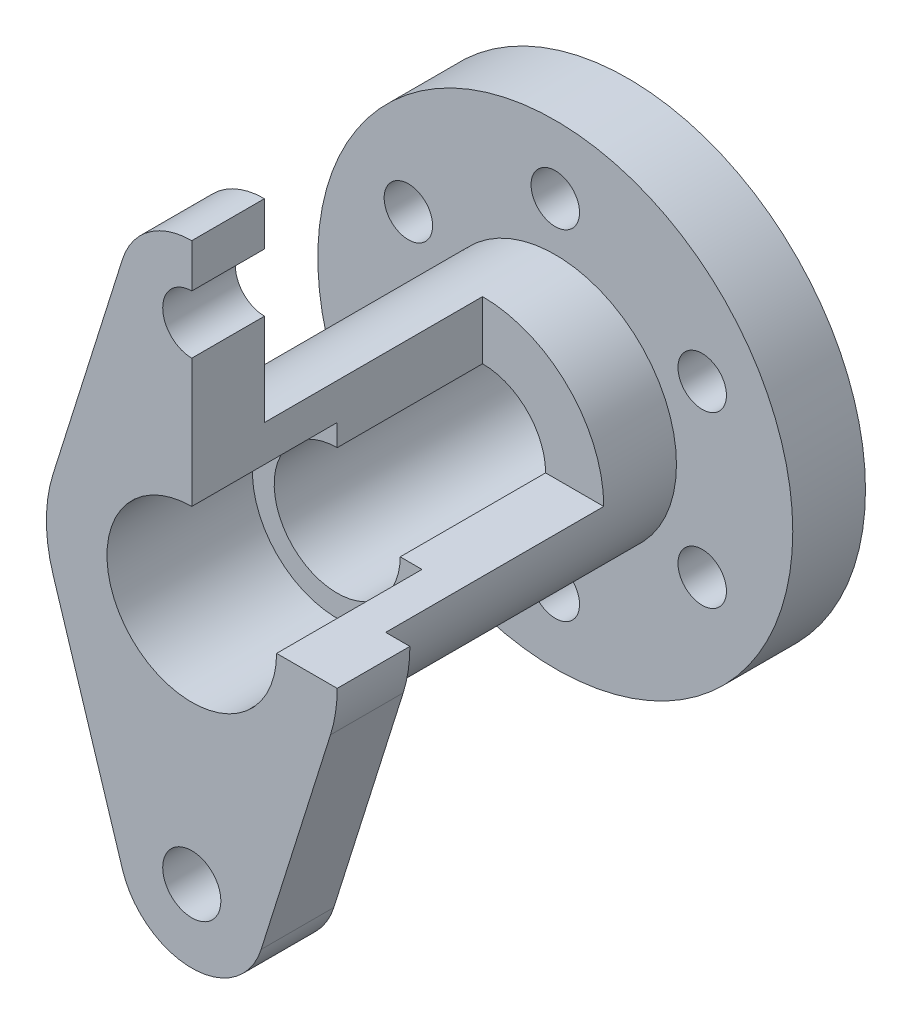
ISO-10303-21;
HEADER;
FILE_DESCRIPTION(('STEP AP214'),'2;1');
FILE_NAME('part.step','',(''),(''),'','','');
FILE_SCHEMA(('AUTOMOTIVE_DESIGN { 1 0 10303 214 1 1 1 1 }'));
ENDSEC;
DATA;
#1=APPLICATION_CONTEXT('core data for automotive mechanical design processes');
#2=APPLICATION_PROTOCOL_DEFINITION('international standard','automotive_design',2000,#1);
#3=PRODUCT_CONTEXT('',#1,'mechanical');
#4=PRODUCT('Part','Part','',(#3));
#5=PRODUCT_RELATED_PRODUCT_CATEGORY('part','',(#4));
#6=PRODUCT_DEFINITION_FORMATION('','',#4);
#7=PRODUCT_DEFINITION_CONTEXT('part definition',#1,'design');
#8=PRODUCT_DEFINITION('design','',#6,#7);
#9=PRODUCT_DEFINITION_SHAPE('','',#8);
#10=(LENGTH_UNIT() NAMED_UNIT(*) SI_UNIT(.MILLI.,.METRE.));
#11=(NAMED_UNIT(*) PLANE_ANGLE_UNIT() SI_UNIT($,.RADIAN.));
#12=(NAMED_UNIT(*) SI_UNIT($,.STERADIAN.) SOLID_ANGLE_UNIT());
#13=UNCERTAINTY_MEASURE_WITH_UNIT(LENGTH_MEASURE(1.E-05),#10,'distance_accuracy_value','');
#14=(GEOMETRIC_REPRESENTATION_CONTEXT(3) GLOBAL_UNCERTAINTY_ASSIGNED_CONTEXT((#13)) GLOBAL_UNIT_ASSIGNED_CONTEXT((#10,
#11,#12)) REPRESENTATION_CONTEXT('',''));
#15=CARTESIAN_POINT('',(0.,0.,0.));
#16=DIRECTION('',(0.,0.,1.));
#17=DIRECTION('',(1.,0.,0.));
#18=AXIS2_PLACEMENT_3D('',#15,#16,#17);
#19=CARTESIAN_POINT('',(0.,65.,15.));
#20=DIRECTION('',(-1.,0.,0.));
#21=DIRECTION('',(0.,-1.,0.));
#22=AXIS2_PLACEMENT_3D('',#19,#20,#21);
#23=PLANE('',#22);
#24=DIRECTION('',(0.,-1.,0.));
#25=VECTOR('',#24,1.);
#26=CARTESIAN_POINT('',(0.,0.,60.));
#27=LINE('',#26,#25);
#28=CARTESIAN_POINT('',(0.,44.,60.));
#29=VERTEX_POINT('',#28);
#30=CARTESIAN_POINT('',(0.,25.,60.));
#31=VERTEX_POINT('',#30);
#32=EDGE_CURVE('E313',#29,#31,#27,.T.);
#33=ORIENTED_EDGE('',*,*,#32,.F.);
#34=DIRECTION('',(0.,0.,1.));
#35=VECTOR('',#34,1.);
#36=CARTESIAN_POINT('',(0.,44.,15.));
#37=LINE('',#36,#35);
#38=CARTESIAN_POINT('',(0.,44.,75.));
#39=VERTEX_POINT('',#38);
#40=EDGE_CURVE('E11',#29,#39,#37,.T.);
#41=ORIENTED_EDGE('',*,*,#40,.T.);
#42=DIRECTION('',(0.,-1.,0.));
#43=VECTOR('',#42,1.);
#44=CARTESIAN_POINT('',(0.,65.,75.));
#45=LINE('',#44,#43);
#46=CARTESIAN_POINT('',(0.,17.5,75.));
#47=VERTEX_POINT('',#46);
#48=EDGE_CURVE('E204',#39,#47,#45,.T.);
#49=ORIENTED_EDGE('',*,*,#48,.T.);
#50=DIRECTION('',(0.,0.,1.));
#51=VECTOR('',#50,1.);
#52=CARTESIAN_POINT('',(0.,17.5,15.));
#53=LINE('',#52,#51);
#54=CARTESIAN_POINT('',(0.,17.5,45.));
#55=VERTEX_POINT('',#54);
#56=EDGE_CURVE('E325',#47,#55,#53,.F.);
#57=ORIENTED_EDGE('',*,*,#56,.T.);
#58=DIRECTION('',(0.,-1.,0.));
#59=VECTOR('',#58,1.);
#60=CARTESIAN_POINT('',(0.,0.,45.));
#61=LINE('',#60,#59);
#62=CARTESIAN_POINT('',(0.,13.,45.));
#63=VERTEX_POINT('',#62);
#64=EDGE_CURVE('E60',#55,#63,#61,.T.);
#65=ORIENTED_EDGE('',*,*,#64,.T.);
#66=DIRECTION('',(0.,0.,-1.));
#67=VECTOR('',#66,1.);
#68=CARTESIAN_POINT('',(0.,13.,45.));
#69=LINE('',#68,#67);
#70=CARTESIAN_POINT('',(0.,13.,15.));
#71=VERTEX_POINT('',#70);
#72=EDGE_CURVE('E182',#63,#71,#69,.T.);
#73=ORIENTED_EDGE('',*,*,#72,.T.);
#74=DIRECTION('',(0.,-1.,0.));
#75=VECTOR('',#74,1.);
#76=CARTESIAN_POINT('',(0.,65.,15.));
#77=LINE('',#76,#75);
#78=CARTESIAN_POINT('',(0.,25.,15.));
#79=VERTEX_POINT('',#78);
#80=EDGE_CURVE('E161',#79,#71,#77,.T.);
#81=ORIENTED_EDGE('',*,*,#80,.F.);
#82=DIRECTION('',(0.,0.,-1.));
#83=VECTOR('',#82,1.);
#84=CARTESIAN_POINT('',(0.,25.,60.));
#85=LINE('',#84,#83);
#86=EDGE_CURVE('E207',#31,#79,#85,.T.);
#87=ORIENTED_EDGE('',*,*,#86,.F.);
#88=EDGE_LOOP('',(#33,#41,#49,#57,#65,#73,#81,#87));
#89=FACE_BOUND('',#88,.T.);
#90=ADVANCED_FACE('F41',(#89),#23,.F.);
#91=CARTESIAN_POINT('',(0.,0.,-15.));
#92=DIRECTION('',(0.,0.,1.));
#93=DIRECTION('',(1.,0.,0.));
#94=AXIS2_PLACEMENT_3D('',#91,#92,#93);
#95=CYLINDRICAL_SURFACE('',#94,49.);
#96=CARTESIAN_POINT('',(0.,0.,-15.));
#97=DIRECTION('',(0.,0.,1.));
#98=DIRECTION('',(1.,0.,0.));
#99=AXIS2_PLACEMENT_3D('',#96,#97,#98);
#100=CIRCLE('',#99,49.);
#101=CARTESIAN_POINT('',(49.,0.,-15.));
#102=VERTEX_POINT('',#101);
#103=EDGE_CURVE('E306',#102,#102,#100,.T.);
#104=ORIENTED_EDGE('',*,*,#103,.T.);
#105=EDGE_LOOP('',(#104));
#106=FACE_BOUND('',#105,.T.);
#107=CARTESIAN_POINT('',(0.,0.,0.));
#108=DIRECTION('',(0.,0.,1.));
#109=DIRECTION('',(1.,0.,0.));
#110=AXIS2_PLACEMENT_3D('',#107,#108,#109);
#111=CIRCLE('',#110,49.);
#112=CARTESIAN_POINT('',(49.,0.,0.));
#113=VERTEX_POINT('',#112);
#114=EDGE_CURVE('E274',#113,#113,#111,.T.);
#115=ORIENTED_EDGE('',*,*,#114,.F.);
#116=EDGE_LOOP('',(#115));
#117=FACE_BOUND('',#116,.T.);
#118=ADVANCED_FACE('F43',(#106,#117),#95,.T.);
#119=CARTESIAN_POINT('',(0.,0.,-15.));
#120=DIRECTION('',(0.,0.,1.));
#121=DIRECTION('',(1.,0.,0.));
#122=AXIS2_PLACEMENT_3D('',#119,#120,#121);
#123=PLANE('',#122);
#124=CARTESIAN_POINT('',(0.,0.,-15.));
#125=DIRECTION('',(0.,0.,1.));
#126=DIRECTION('',(1.,0.,0.));
#127=AXIS2_PLACEMENT_3D('',#124,#125,#126);
#128=CIRCLE('',#127,13.);
#129=CARTESIAN_POINT('',(13.,0.,-15.));
#130=VERTEX_POINT('',#129);
#131=EDGE_CURVE('E164',#130,#130,#128,.T.);
#132=ORIENTED_EDGE('',*,*,#131,.T.);
#133=EDGE_LOOP('',(#132));
#134=FACE_BOUND('',#133,.T.);
#135=CARTESIAN_POINT('',(0.,35.,-15.));
#136=DIRECTION('',(0.,0.,1.));
#137=DIRECTION('',(1.,0.,0.));
#138=AXIS2_PLACEMENT_3D('',#135,#136,#137);
#139=CIRCLE('',#138,5.);
#140=CARTESIAN_POINT('',(5.,35.,-15.));
#141=VERTEX_POINT('',#140);
#142=EDGE_CURVE('E275',#141,#141,#139,.T.);
#143=ORIENTED_EDGE('',*,*,#142,.T.);
#144=EDGE_LOOP('',(#143));
#145=FACE_BOUND('',#144,.T.);
#146=CARTESIAN_POINT('',(-30.3108891324546,17.4999999999987,-15.));
#147=DIRECTION('',(0.,0.,1.));
#148=DIRECTION('',(1.,0.,0.));
#149=AXIS2_PLACEMENT_3D('',#146,#147,#148);
#150=CIRCLE('',#149,5.0000000000015);
#151=CARTESIAN_POINT('',(-25.3108891324531,17.4999999999987,-15.));
#152=VERTEX_POINT('',#151);
#153=EDGE_CURVE('E278',#152,#152,#150,.T.);
#154=ORIENTED_EDGE('',*,*,#153,.T.);
#155=EDGE_LOOP('',(#154));
#156=FACE_BOUND('',#155,.T.);
#157=CARTESIAN_POINT('',(-30.3108891324531,-17.5000000000013,-15.));
#158=DIRECTION('',(0.,0.,1.));
#159=DIRECTION('',(1.,0.,0.));
#160=AXIS2_PLACEMENT_3D('',#157,#158,#159);
#161=CIRCLE('',#160,5.00000000000282);
#162=CARTESIAN_POINT('',(-25.3108891324503,-17.5000000000013,-15.));
#163=VERTEX_POINT('',#162);
#164=EDGE_CURVE('E302',#163,#163,#161,.T.);
#165=ORIENTED_EDGE('',*,*,#164,.T.);
#166=EDGE_LOOP('',(#165));
#167=FACE_BOUND('',#166,.T.);
#168=CARTESIAN_POINT('',(2.97142069880137E-12,-35.,-15.));
#169=DIRECTION('',(0.,0.,1.));
#170=DIRECTION('',(1.,0.,0.));
#171=AXIS2_PLACEMENT_3D('',#168,#169,#170);
#172=CIRCLE('',#171,5.00000000000307);
#173=CARTESIAN_POINT('',(5.00000000000605,-35.,-15.));
#174=VERTEX_POINT('',#173);
#175=EDGE_CURVE('E297',#174,#174,#172,.T.);
#176=ORIENTED_EDGE('',*,*,#175,.T.);
#177=EDGE_LOOP('',(#176));
#178=FACE_BOUND('',#177,.T.);
#179=CARTESIAN_POINT('',(30.3108891324576,-17.4999999999987,-15.));
#180=DIRECTION('',(0.,0.,1.));
#181=DIRECTION('',(1.,0.,0.));
#182=AXIS2_PLACEMENT_3D('',#179,#180,#181);
#183=CIRCLE('',#182,5.00000000000192);
#184=CARTESIAN_POINT('',(35.3108891324595,-17.4999999999987,-15.));
#185=VERTEX_POINT('',#184);
#186=EDGE_CURVE('E292',#185,#185,#183,.T.);
#187=ORIENTED_EDGE('',*,*,#186,.T.);
#188=EDGE_LOOP('',(#187));
#189=FACE_BOUND('',#188,.T.);
#190=CARTESIAN_POINT('',(30.3108891324561,17.5000000000013,-15.));
#191=DIRECTION('',(0.,0.,1.));
#192=DIRECTION('',(1.,0.,0.));
#193=AXIS2_PLACEMENT_3D('',#190,#191,#192);
#194=CIRCLE('',#193,5.0000000000004);
#195=CARTESIAN_POINT('',(35.3108891324565,17.5000000000013,-15.));
#196=VERTEX_POINT('',#195);
#197=EDGE_CURVE('E276',#196,#196,#194,.T.);
#198=ORIENTED_EDGE('',*,*,#197,.T.);
#199=EDGE_LOOP('',(#198));
#200=FACE_BOUND('',#199,.T.);
#201=ORIENTED_EDGE('',*,*,#103,.F.);
#202=EDGE_LOOP('',(#201));
#203=FACE_BOUND('',#202,.T.);
#204=ADVANCED_FACE('F401',(#134,#145,#156,#167,#178,#189,#200,#203),#123,.F.);
#205=CARTESIAN_POINT('',(0.,0.,0.));
#206=DIRECTION('',(0.,0.,1.));
#207=DIRECTION('',(1.,0.,0.));
#208=AXIS2_PLACEMENT_3D('',#205,#206,#207);
#209=PLANE('',#208);
#210=CARTESIAN_POINT('',(0.,0.,0.));
#211=DIRECTION('',(0.,0.,1.));
#212=DIRECTION('',(1.,0.,0.));
#213=AXIS2_PLACEMENT_3D('',#210,#211,#212);
#214=CIRCLE('',#213,25.);
#215=CARTESIAN_POINT('',(25.,0.,0.));
#216=VERTEX_POINT('',#215);
#217=EDGE_CURVE('E264',#216,#216,#214,.T.);
#218=ORIENTED_EDGE('',*,*,#217,.F.);
#219=EDGE_LOOP('',(#218));
#220=FACE_BOUND('',#219,.T.);
#221=CARTESIAN_POINT('',(0.,35.,0.));
#222=DIRECTION('',(0.,0.,1.));
#223=DIRECTION('',(1.,0.,0.));
#224=AXIS2_PLACEMENT_3D('',#221,#222,#223);
#225=CIRCLE('',#224,5.);
#226=CARTESIAN_POINT('',(5.,35.,0.));
#227=VERTEX_POINT('',#226);
#228=EDGE_CURVE('E277',#227,#227,#225,.T.);
#229=ORIENTED_EDGE('',*,*,#228,.F.);
#230=EDGE_LOOP('',(#229));
#231=FACE_BOUND('',#230,.T.);
#232=CARTESIAN_POINT('',(-30.3108891324546,17.4999999999987,0.));
#233=DIRECTION('',(0.,0.,1.));
#234=DIRECTION('',(1.,0.,0.));
#235=AXIS2_PLACEMENT_3D('',#232,#233,#234);
#236=CIRCLE('',#235,5.0000000000015);
#237=CARTESIAN_POINT('',(-25.3108891324531,17.4999999999987,0.));
#238=VERTEX_POINT('',#237);
#239=EDGE_CURVE('E267',#238,#238,#236,.T.);
#240=ORIENTED_EDGE('',*,*,#239,.F.);
#241=EDGE_LOOP('',(#240));
#242=FACE_BOUND('',#241,.T.);
#243=CARTESIAN_POINT('',(-30.3108891324531,-17.5000000000013,0.));
#244=DIRECTION('',(0.,0.,1.));
#245=DIRECTION('',(1.,0.,0.));
#246=AXIS2_PLACEMENT_3D('',#243,#244,#245);
#247=CIRCLE('',#246,5.00000000000282);
#248=CARTESIAN_POINT('',(-25.3108891324503,-17.5000000000013,0.));
#249=VERTEX_POINT('',#248);
#250=EDGE_CURVE('E284',#249,#249,#247,.T.);
#251=ORIENTED_EDGE('',*,*,#250,.F.);
#252=EDGE_LOOP('',(#251));
#253=FACE_BOUND('',#252,.T.);
#254=CARTESIAN_POINT('',(2.97142069880137E-12,-35.,0.));
#255=DIRECTION('',(0.,0.,1.));
#256=DIRECTION('',(1.,0.,0.));
#257=AXIS2_PLACEMENT_3D('',#254,#255,#256);
#258=CIRCLE('',#257,5.00000000000307);
#259=CARTESIAN_POINT('',(5.00000000000605,-35.,0.));
#260=VERTEX_POINT('',#259);
#261=EDGE_CURVE('E300',#260,#260,#258,.T.);
#262=ORIENTED_EDGE('',*,*,#261,.F.);
#263=EDGE_LOOP('',(#262));
#264=FACE_BOUND('',#263,.T.);
#265=CARTESIAN_POINT('',(30.3108891324576,-17.4999999999987,0.));
#266=DIRECTION('',(0.,0.,1.));
#267=DIRECTION('',(1.,0.,0.));
#268=AXIS2_PLACEMENT_3D('',#265,#266,#267);
#269=CIRCLE('',#268,5.00000000000192);
#270=CARTESIAN_POINT('',(35.3108891324595,-17.4999999999987,0.));
#271=VERTEX_POINT('',#270);
#272=EDGE_CURVE('E294',#271,#271,#269,.T.);
#273=ORIENTED_EDGE('',*,*,#272,.F.);
#274=EDGE_LOOP('',(#273));
#275=FACE_BOUND('',#274,.T.);
#276=CARTESIAN_POINT('',(30.3108891324561,17.5000000000013,0.));
#277=DIRECTION('',(0.,0.,1.));
#278=DIRECTION('',(1.,0.,0.));
#279=AXIS2_PLACEMENT_3D('',#276,#277,#278);
#280=CIRCLE('',#279,5.0000000000004);
#281=CARTESIAN_POINT('',(35.3108891324565,17.5000000000013,0.));
#282=VERTEX_POINT('',#281);
#283=EDGE_CURVE('E287',#282,#282,#280,.T.);
#284=ORIENTED_EDGE('',*,*,#283,.F.);
#285=EDGE_LOOP('',(#284));
#286=FACE_BOUND('',#285,.T.);
#287=ORIENTED_EDGE('',*,*,#114,.T.);
#288=EDGE_LOOP('',(#287));
#289=FACE_BOUND('',#288,.T.);
#290=ADVANCED_FACE('F552',(#220,#231,#242,#253,#264,#275,#286,#289),#209,.T.);
#291=CARTESIAN_POINT('',(30.3108891324561,17.5000000000013,-15.));
#292=DIRECTION('',(0.,0.,1.));
#293=DIRECTION('',(1.,0.,0.));
#294=AXIS2_PLACEMENT_3D('',#291,#292,#293);
#295=CYLINDRICAL_SURFACE('',#294,5.0000000000004);
#296=ORIENTED_EDGE('',*,*,#197,.F.);
#297=EDGE_LOOP('',(#296));
#298=FACE_BOUND('',#297,.T.);
#299=ORIENTED_EDGE('',*,*,#283,.T.);
#300=EDGE_LOOP('',(#299));
#301=FACE_BOUND('',#300,.T.);
#302=ADVANCED_FACE('F570',(#298,#301),#295,.F.);
#303=CARTESIAN_POINT('',(30.3108891324576,-17.4999999999987,-15.));
#304=DIRECTION('',(0.,0.,1.));
#305=DIRECTION('',(1.,0.,0.));
#306=AXIS2_PLACEMENT_3D('',#303,#304,#305);
#307=CYLINDRICAL_SURFACE('',#306,5.00000000000192);
#308=ORIENTED_EDGE('',*,*,#186,.F.);
#309=EDGE_LOOP('',(#308));
#310=FACE_BOUND('',#309,.T.);
#311=ORIENTED_EDGE('',*,*,#272,.T.);
#312=EDGE_LOOP('',(#311));
#313=FACE_BOUND('',#312,.T.);
#314=ADVANCED_FACE('F580',(#310,#313),#307,.F.);
#315=CARTESIAN_POINT('',(2.97142069880137E-12,-35.,-15.));
#316=DIRECTION('',(0.,0.,1.));
#317=DIRECTION('',(1.,0.,0.));
#318=AXIS2_PLACEMENT_3D('',#315,#316,#317);
#319=CYLINDRICAL_SURFACE('',#318,5.00000000000307);
#320=ORIENTED_EDGE('',*,*,#175,.F.);
#321=EDGE_LOOP('',(#320));
#322=FACE_BOUND('',#321,.T.);
#323=ORIENTED_EDGE('',*,*,#261,.T.);
#324=EDGE_LOOP('',(#323));
#325=FACE_BOUND('',#324,.T.);
#326=ADVANCED_FACE('F590',(#322,#325),#319,.F.);
#327=CARTESIAN_POINT('',(-30.3108891324531,-17.5000000000013,-15.));
#328=DIRECTION('',(0.,0.,1.));
#329=DIRECTION('',(1.,0.,0.));
#330=AXIS2_PLACEMENT_3D('',#327,#328,#329);
#331=CYLINDRICAL_SURFACE('',#330,5.00000000000282);
#332=ORIENTED_EDGE('',*,*,#164,.F.);
#333=EDGE_LOOP('',(#332));
#334=FACE_BOUND('',#333,.T.);
#335=ORIENTED_EDGE('',*,*,#250,.T.);
#336=EDGE_LOOP('',(#335));
#337=FACE_BOUND('',#336,.T.);
#338=ADVANCED_FACE('F600',(#334,#337),#331,.F.);
#339=CARTESIAN_POINT('',(-30.3108891324546,17.4999999999987,-15.));
#340=DIRECTION('',(0.,0.,1.));
#341=DIRECTION('',(1.,0.,0.));
#342=AXIS2_PLACEMENT_3D('',#339,#340,#341);
#343=CYLINDRICAL_SURFACE('',#342,5.0000000000015);
#344=ORIENTED_EDGE('',*,*,#153,.F.);
#345=EDGE_LOOP('',(#344));
#346=FACE_BOUND('',#345,.T.);
#347=ORIENTED_EDGE('',*,*,#239,.T.);
#348=EDGE_LOOP('',(#347));
#349=FACE_BOUND('',#348,.T.);
#350=ADVANCED_FACE('F610',(#346,#349),#343,.F.);
#351=CARTESIAN_POINT('',(0.,35.,-15.));
#352=DIRECTION('',(0.,0.,1.));
#353=DIRECTION('',(1.,0.,0.));
#354=AXIS2_PLACEMENT_3D('',#351,#352,#353);
#355=CYLINDRICAL_SURFACE('',#354,5.);
#356=ORIENTED_EDGE('',*,*,#142,.F.);
#357=EDGE_LOOP('',(#356));
#358=FACE_BOUND('',#357,.T.);
#359=ORIENTED_EDGE('',*,*,#228,.T.);
#360=EDGE_LOOP('',(#359));
#361=FACE_BOUND('',#360,.T.);
#362=ADVANCED_FACE('F393',(#358,#361),#355,.F.);
#363=CARTESIAN_POINT('',(0.,0.,60.));
#364=DIRECTION('',(0.,0.,-1.));
#365=DIRECTION('',(-1.,0.,0.));
#366=AXIS2_PLACEMENT_3D('',#363,#364,#365);
#367=CYLINDRICAL_SURFACE('',#366,25.);
#368=CARTESIAN_POINT('',(0.,0.,15.));
#369=DIRECTION('',(0.,0.,-1.));
#370=DIRECTION('',(-1.,0.,0.));
#371=AXIS2_PLACEMENT_3D('',#368,#369,#370);
#372=CIRCLE('',#371,25.);
#373=CARTESIAN_POINT('',(25.,0.,15.));
#374=VERTEX_POINT('',#373);
#375=EDGE_CURVE('E319',#79,#374,#372,.T.);
#376=ORIENTED_EDGE('',*,*,#375,.T.);
#377=DIRECTION('',(0.,0.,-1.));
#378=VECTOR('',#377,1.);
#379=CARTESIAN_POINT('',(25.,0.,60.));
#380=LINE('',#379,#378);
#381=CARTESIAN_POINT('',(25.,0.,60.));
#382=VERTEX_POINT('',#381);
#383=EDGE_CURVE('E174',#374,#382,#380,.F.);
#384=ORIENTED_EDGE('',*,*,#383,.T.);
#385=CARTESIAN_POINT('',(0.,0.,60.));
#386=DIRECTION('',(0.,0.,1.));
#387=DIRECTION('',(1.,0.,0.));
#388=AXIS2_PLACEMENT_3D('',#385,#386,#387);
#389=CIRCLE('',#388,25.);
#390=EDGE_CURVE('E266',#31,#382,#389,.T.);
#391=ORIENTED_EDGE('',*,*,#390,.F.);
#392=ORIENTED_EDGE('',*,*,#86,.T.);
#393=EDGE_LOOP('',(#376,#384,#391,#392));
#394=FACE_BOUND('',#393,.T.);
#395=ORIENTED_EDGE('',*,*,#217,.T.);
#396=EDGE_LOOP('',(#395));
#397=FACE_BOUND('',#396,.T.);
#398=ADVANCED_FACE('F360',(#394,#397),#367,.T.);
#399=CARTESIAN_POINT('',(0.,0.,75.));
#400=DIRECTION('',(0.,0.,-1.));
#401=DIRECTION('',(-1.,0.,0.));
#402=AXIS2_PLACEMENT_3D('',#399,#400,#401);
#403=CYLINDRICAL_SURFACE('',#402,30.);
#404=CARTESIAN_POINT('',(0.,0.,60.));
#405=DIRECTION('',(0.,0.,1.));
#406=DIRECTION('',(1.,0.,0.));
#407=AXIS2_PLACEMENT_3D('',#404,#405,#406);
#408=CIRCLE('',#407,30.);
#409=CARTESIAN_POINT('',(-28.6181760425084,9.,60.));
#410=VERTEX_POINT('',#409);
#411=CARTESIAN_POINT('',(-28.6181760425084,-9.,60.));
#412=VERTEX_POINT('',#411);
#413=EDGE_CURVE('E214',#410,#412,#408,.T.);
#414=ORIENTED_EDGE('',*,*,#413,.T.);
#415=DIRECTION('',(0.,0.,-1.));
#416=VECTOR('',#415,1.);
#417=CARTESIAN_POINT('',(-28.6181760425084,-9.,75.));
#418=LINE('',#417,#416);
#419=CARTESIAN_POINT('',(-28.6181760425084,-9.,75.));
#420=VERTEX_POINT('',#419);
#421=EDGE_CURVE('E265',#420,#412,#418,.T.);
#422=ORIENTED_EDGE('',*,*,#421,.F.);
#423=CARTESIAN_POINT('',(0.,0.,75.));
#424=DIRECTION('',(0.,0.,1.));
#425=DIRECTION('',(1.,0.,0.));
#426=AXIS2_PLACEMENT_3D('',#423,#424,#425);
#427=CIRCLE('',#426,30.);
#428=CARTESIAN_POINT('',(-28.6181760425084,9.,75.));
#429=VERTEX_POINT('',#428);
#430=EDGE_CURVE('E216',#429,#420,#427,.T.);
#431=ORIENTED_EDGE('',*,*,#430,.F.);
#432=DIRECTION('',(0.,0.,-1.));
#433=VECTOR('',#432,1.);
#434=CARTESIAN_POINT('',(-28.6181760425084,9.,75.));
#435=LINE('',#434,#433);
#436=EDGE_CURVE('E232',#429,#410,#435,.T.);
#437=ORIENTED_EDGE('',*,*,#436,.T.);
#438=EDGE_LOOP('',(#414,#422,#431,#437));
#439=FACE_BOUND('',#438,.T.);
#440=ADVANCED_FACE('F384',(#439),#403,.T.);
#441=CARTESIAN_POINT('',(-28.6181760425084,-9.,75.));
#442=DIRECTION('',(0.953939201416946,0.3,0.));
#443=DIRECTION('',(-0.3,0.953939201416946,0.));
#444=AXIS2_PLACEMENT_3D('',#441,#442,#443);
#445=PLANE('',#444);
#446=DIRECTION('',(0.3,-0.953939201416946,0.));
#447=VECTOR('',#446,1.);
#448=CARTESIAN_POINT('',(-28.6181760425084,-9.,60.));
#449=LINE('',#448,#447);
#450=CARTESIAN_POINT('',(-14.3090880212542,-54.5,60.));
#451=VERTEX_POINT('',#450);
#452=EDGE_CURVE('E237',#412,#451,#449,.T.);
#453=ORIENTED_EDGE('',*,*,#452,.T.);
#454=DIRECTION('',(0.,0.,-1.));
#455=VECTOR('',#454,1.);
#456=CARTESIAN_POINT('',(-14.3090880212542,-54.5,75.));
#457=LINE('',#456,#455);
#458=CARTESIAN_POINT('',(-14.3090880212542,-54.5,75.));
#459=VERTEX_POINT('',#458);
#460=EDGE_CURVE('E259',#459,#451,#457,.T.);
#461=ORIENTED_EDGE('',*,*,#460,.F.);
#462=DIRECTION('',(0.3,-0.953939201416946,0.));
#463=VECTOR('',#462,1.);
#464=CARTESIAN_POINT('',(-28.6181760425084,-9.,75.));
#465=LINE('',#464,#463);
#466=EDGE_CURVE('E218',#420,#459,#465,.T.);
#467=ORIENTED_EDGE('',*,*,#466,.F.);
#468=ORIENTED_EDGE('',*,*,#421,.T.);
#469=EDGE_LOOP('',(#453,#461,#467,#468));
#470=FACE_BOUND('',#469,.T.);
#471=ADVANCED_FACE('F382',(#470),#445,.F.);
#472=CARTESIAN_POINT('',(0.,-50.,75.));
#473=DIRECTION('',(0.,0.,-1.));
#474=DIRECTION('',(-1.,0.,0.));
#475=AXIS2_PLACEMENT_3D('',#472,#473,#474);
#476=CYLINDRICAL_SURFACE('',#475,15.);
#477=CARTESIAN_POINT('',(0.,-50.,60.));
#478=DIRECTION('',(0.,0.,1.));
#479=DIRECTION('',(1.,0.,0.));
#480=AXIS2_PLACEMENT_3D('',#477,#478,#479);
#481=CIRCLE('',#480,15.);
#482=CARTESIAN_POINT('',(14.3090880212542,-54.5,60.));
#483=VERTEX_POINT('',#482);
#484=EDGE_CURVE('E236',#451,#483,#481,.T.);
#485=ORIENTED_EDGE('',*,*,#484,.T.);
#486=DIRECTION('',(0.,0.,-1.));
#487=VECTOR('',#486,1.);
#488=CARTESIAN_POINT('',(14.3090880212542,-54.5,75.));
#489=LINE('',#488,#487);
#490=CARTESIAN_POINT('',(14.3090880212542,-54.5,75.));
#491=VERTEX_POINT('',#490);
#492=EDGE_CURVE('E258',#491,#483,#489,.T.);
#493=ORIENTED_EDGE('',*,*,#492,.F.);
#494=CARTESIAN_POINT('',(0.,-50.,75.));
#495=DIRECTION('',(0.,0.,1.));
#496=DIRECTION('',(1.,0.,0.));
#497=AXIS2_PLACEMENT_3D('',#494,#495,#496);
#498=CIRCLE('',#497,15.);
#499=EDGE_CURVE('E225',#459,#491,#498,.T.);
#500=ORIENTED_EDGE('',*,*,#499,.F.);
#501=ORIENTED_EDGE('',*,*,#460,.T.);
#502=EDGE_LOOP('',(#485,#493,#500,#501));
#503=FACE_BOUND('',#502,.T.);
#504=ADVANCED_FACE('F379',(#503),#476,.T.);
#505=CARTESIAN_POINT('',(28.6181760425084,-8.99999999999999,75.));
#506=DIRECTION('',(-0.953939201416946,0.3,0.));
#507=DIRECTION('',(-0.3,-0.953939201416946,0.));
#508=AXIS2_PLACEMENT_3D('',#505,#506,#507);
#509=PLANE('',#508);
#510=DIRECTION('',(0.3,0.953939201416946,0.));
#511=VECTOR('',#510,1.);
#512=CARTESIAN_POINT('',(28.6181760425084,-8.99999999999999,60.));
#513=LINE('',#512,#511);
#514=CARTESIAN_POINT('',(28.6181760425084,-8.99999999999999,60.));
#515=VERTEX_POINT('',#514);
#516=EDGE_CURVE('E238',#483,#515,#513,.T.);
#517=ORIENTED_EDGE('',*,*,#516,.T.);
#518=DIRECTION('',(0.,0.,-1.));
#519=VECTOR('',#518,1.);
#520=CARTESIAN_POINT('',(28.6181760425084,-8.99999999999999,75.));
#521=LINE('',#520,#519);
#522=CARTESIAN_POINT('',(28.6181760425084,-8.99999999999999,75.));
#523=VERTEX_POINT('',#522);
#524=EDGE_CURVE('E251',#523,#515,#521,.T.);
#525=ORIENTED_EDGE('',*,*,#524,.F.);
#526=DIRECTION('',(0.3,0.953939201416946,0.));
#527=VECTOR('',#526,1.);
#528=CARTESIAN_POINT('',(28.6181760425084,-8.99999999999999,75.));
#529=LINE('',#528,#527);
#530=EDGE_CURVE('E221',#491,#523,#529,.T.);
#531=ORIENTED_EDGE('',*,*,#530,.F.);
#532=ORIENTED_EDGE('',*,*,#492,.T.);
#533=EDGE_LOOP('',(#517,#525,#531,#532));
#534=FACE_BOUND('',#533,.T.);
#535=ADVANCED_FACE('F374',(#534),#509,.F.);
#536=CARTESIAN_POINT('',(0.,0.,75.));
#537=DIRECTION('',(0.,0.,-1.));
#538=DIRECTION('',(-1.,0.,0.));
#539=AXIS2_PLACEMENT_3D('',#536,#537,#538);
#540=CYLINDRICAL_SURFACE('',#539,30.);
#541=CARTESIAN_POINT('',(0.,0.,60.));
#542=DIRECTION('',(0.,0.,1.));
#543=DIRECTION('',(1.,0.,0.));
#544=AXIS2_PLACEMENT_3D('',#541,#542,#543);
#545=CIRCLE('',#544,30.);
#546=CARTESIAN_POINT('',(30.,0.,60.));
#547=VERTEX_POINT('',#546);
#548=EDGE_CURVE('E242',#515,#547,#545,.T.);
#549=ORIENTED_EDGE('',*,*,#548,.T.);
#550=DIRECTION('',(0.,0.,1.));
#551=VECTOR('',#550,1.);
#552=CARTESIAN_POINT('',(30.,0.,15.));
#553=LINE('',#552,#551);
#554=CARTESIAN_POINT('',(30.,0.,75.));
#555=VERTEX_POINT('',#554);
#556=EDGE_CURVE('E203',#547,#555,#553,.T.);
#557=ORIENTED_EDGE('',*,*,#556,.T.);
#558=CARTESIAN_POINT('',(0.,0.,75.));
#559=DIRECTION('',(0.,0.,1.));
#560=DIRECTION('',(1.,0.,0.));
#561=AXIS2_PLACEMENT_3D('',#558,#559,#560);
#562=CIRCLE('',#561,30.);
#563=EDGE_CURVE('E226',#523,#555,#562,.T.);
#564=ORIENTED_EDGE('',*,*,#563,.F.);
#565=ORIENTED_EDGE('',*,*,#524,.T.);
#566=EDGE_LOOP('',(#549,#557,#564,#565));
#567=FACE_BOUND('',#566,.T.);
#568=ADVANCED_FACE('F367',(#567),#540,.T.);
#569=CARTESIAN_POINT('',(0.,50.,75.));
#570=DIRECTION('',(0.,0.,-1.));
#571=DIRECTION('',(-1.,0.,0.));
#572=AXIS2_PLACEMENT_3D('',#569,#570,#571);
#573=CYLINDRICAL_SURFACE('',#572,15.);
#574=CARTESIAN_POINT('',(0.,50.,75.));
#575=DIRECTION('',(0.,0.,1.));
#576=DIRECTION('',(-1.,0.,0.));
#577=AXIS2_PLACEMENT_3D('',#574,#575,#576);
#578=CIRCLE('',#577,15.);
#579=CARTESIAN_POINT('',(0.,65.,75.));
#580=VERTEX_POINT('',#579);
#581=CARTESIAN_POINT('',(-14.3090880212542,54.5,75.));
#582=VERTEX_POINT('',#581);
#583=EDGE_CURVE('E228',#580,#582,#578,.T.);
#584=ORIENTED_EDGE('',*,*,#583,.F.);
#585=DIRECTION('',(0.,0.,1.));
#586=VECTOR('',#585,1.);
#587=CARTESIAN_POINT('',(0.,65.,15.));
#588=LINE('',#587,#586);
#589=CARTESIAN_POINT('',(0.,65.,60.));
#590=VERTEX_POINT('',#589);
#591=EDGE_CURVE('E210',#590,#580,#588,.T.);
#592=ORIENTED_EDGE('',*,*,#591,.F.);
#593=CARTESIAN_POINT('',(0.,50.,60.));
#594=DIRECTION('',(0.,0.,1.));
#595=DIRECTION('',(-1.,0.,0.));
#596=AXIS2_PLACEMENT_3D('',#593,#594,#595);
#597=CIRCLE('',#596,15.);
#598=CARTESIAN_POINT('',(-14.3090880212542,54.5,60.));
#599=VERTEX_POINT('',#598);
#600=EDGE_CURVE('E245',#590,#599,#597,.T.);
#601=ORIENTED_EDGE('',*,*,#600,.T.);
#602=DIRECTION('',(0.,0.,-1.));
#603=VECTOR('',#602,1.);
#604=CARTESIAN_POINT('',(-14.3090880212542,54.5,75.));
#605=LINE('',#604,#603);
#606=EDGE_CURVE('E249',#582,#599,#605,.T.);
#607=ORIENTED_EDGE('',*,*,#606,.F.);
#608=EDGE_LOOP('',(#584,#592,#601,#607));
#609=FACE_BOUND('',#608,.T.);
#610=ADVANCED_FACE('F338',(#609),#573,.T.);
#611=CARTESIAN_POINT('',(-28.6181760425084,9.,75.));
#612=DIRECTION('',(0.953939201416946,-0.3,0.));
#613=DIRECTION('',(0.3,0.953939201416946,0.));
#614=AXIS2_PLACEMENT_3D('',#611,#612,#613);
#615=PLANE('',#614);
#616=DIRECTION('',(-0.3,-0.953939201416946,0.));
#617=VECTOR('',#616,1.);
#618=CARTESIAN_POINT('',(-28.6181760425084,9.,60.));
#619=LINE('',#618,#617);
#620=EDGE_CURVE('E219',#599,#410,#619,.T.);
#621=ORIENTED_EDGE('',*,*,#620,.T.);
#622=ORIENTED_EDGE('',*,*,#436,.F.);
#623=DIRECTION('',(-0.3,-0.953939201416946,0.));
#624=VECTOR('',#623,1.);
#625=CARTESIAN_POINT('',(-28.6181760425084,9.,75.));
#626=LINE('',#625,#624);
#627=EDGE_CURVE('E231',#582,#429,#626,.T.);
#628=ORIENTED_EDGE('',*,*,#627,.F.);
#629=ORIENTED_EDGE('',*,*,#606,.T.);
#630=EDGE_LOOP('',(#621,#622,#628,#629));
#631=FACE_BOUND('',#630,.T.);
#632=ADVANCED_FACE('F345',(#631),#615,.F.);
#633=CARTESIAN_POINT('',(0.,0.,75.));
#634=DIRECTION('',(0.,0.,1.));
#635=DIRECTION('',(1.,0.,0.));
#636=AXIS2_PLACEMENT_3D('',#633,#634,#635);
#637=PLANE('',#636);
#638=CARTESIAN_POINT('',(0.,-50.,75.));
#639=DIRECTION('',(0.,0.,1.));
#640=DIRECTION('',(-1.,0.,0.));
#641=AXIS2_PLACEMENT_3D('',#638,#639,#640);
#642=CIRCLE('',#641,6.);
#643=CARTESIAN_POINT('',(-5.99999999999998,-50.,75.));
#644=VERTEX_POINT('',#643);
#645=EDGE_CURVE('E184',#644,#644,#642,.T.);
#646=ORIENTED_EDGE('',*,*,#645,.F.);
#647=EDGE_LOOP('',(#646));
#648=FACE_BOUND('',#647,.T.);
#649=CARTESIAN_POINT('',(0.,50.,75.));
#650=DIRECTION('',(0.,0.,1.));
#651=DIRECTION('',(1.,0.,0.));
#652=AXIS2_PLACEMENT_3D('',#649,#650,#651);
#653=CIRCLE('',#652,6.);
#654=CARTESIAN_POINT('',(0.,56.,75.));
#655=VERTEX_POINT('',#654);
#656=EDGE_CURVE('E190',#655,#39,#653,.T.);
#657=ORIENTED_EDGE('',*,*,#656,.F.);
#658=EDGE_CURVE('E175',#580,#655,#45,.T.);
#659=ORIENTED_EDGE('',*,*,#658,.F.);
#660=ORIENTED_EDGE('',*,*,#583,.T.);
#661=ORIENTED_EDGE('',*,*,#627,.T.);
#662=ORIENTED_EDGE('',*,*,#430,.T.);
#663=ORIENTED_EDGE('',*,*,#466,.T.);
#664=ORIENTED_EDGE('',*,*,#499,.T.);
#665=ORIENTED_EDGE('',*,*,#530,.T.);
#666=ORIENTED_EDGE('',*,*,#563,.T.);
#667=DIRECTION('',(1.,0.,0.));
#668=VECTOR('',#667,1.);
#669=CARTESIAN_POINT('',(0.,0.,75.));
#670=LINE('',#669,#668);
#671=CARTESIAN_POINT('',(17.5,0.,75.));
#672=VERTEX_POINT('',#671);
#673=EDGE_CURVE('E205',#672,#555,#670,.T.);
#674=ORIENTED_EDGE('',*,*,#673,.F.);
#675=CARTESIAN_POINT('',(0.,0.,75.));
#676=DIRECTION('',(0.,0.,1.));
#677=DIRECTION('',(1.,0.,0.));
#678=AXIS2_PLACEMENT_3D('',#675,#676,#677);
#679=CIRCLE('',#678,17.5);
#680=EDGE_CURVE('E195',#47,#672,#679,.T.);
#681=ORIENTED_EDGE('',*,*,#680,.F.);
#682=ORIENTED_EDGE('',*,*,#48,.F.);
#683=EDGE_LOOP('',(#657,#659,#660,#661,#662,#663,#664,#665,#666,#674,#681,#682));
#684=FACE_BOUND('',#683,.T.);
#685=ADVANCED_FACE('F347',(#648,#684),#637,.T.);
#686=CARTESIAN_POINT('',(0.,0.,60.));
#687=DIRECTION('',(0.,0.,1.));
#688=DIRECTION('',(1.,0.,0.));
#689=AXIS2_PLACEMENT_3D('',#686,#687,#688);
#690=PLANE('',#689);
#691=CARTESIAN_POINT('',(0.,-50.,60.));
#692=DIRECTION('',(0.,0.,1.));
#693=DIRECTION('',(1.,0.,0.));
#694=AXIS2_PLACEMENT_3D('',#691,#692,#693);
#695=CIRCLE('',#694,6.);
#696=CARTESIAN_POINT('',(6.00000000000002,-50.,60.));
#697=VERTEX_POINT('',#696);
#698=EDGE_CURVE('E44',#697,#697,#695,.T.);
#699=ORIENTED_EDGE('',*,*,#698,.T.);
#700=EDGE_LOOP('',(#699));
#701=FACE_BOUND('',#700,.T.);
#702=CARTESIAN_POINT('',(0.,56.,60.));
#703=VERTEX_POINT('',#702);
#704=EDGE_CURVE('E314',#590,#703,#27,.T.);
#705=ORIENTED_EDGE('',*,*,#704,.T.);
#706=CARTESIAN_POINT('',(0.,50.,60.));
#707=DIRECTION('',(0.,0.,1.));
#708=DIRECTION('',(1.,0.,0.));
#709=AXIS2_PLACEMENT_3D('',#706,#707,#708);
#710=CIRCLE('',#709,6.);
#711=EDGE_CURVE('E65',#703,#29,#710,.T.);
#712=ORIENTED_EDGE('',*,*,#711,.T.);
#713=ORIENTED_EDGE('',*,*,#32,.T.);
#714=ORIENTED_EDGE('',*,*,#390,.T.);
#715=DIRECTION('',(1.,0.,0.));
#716=VECTOR('',#715,1.);
#717=CARTESIAN_POINT('',(0.,0.,60.));
#718=LINE('',#717,#716);
#719=EDGE_CURVE('E320',#382,#547,#718,.T.);
#720=ORIENTED_EDGE('',*,*,#719,.T.);
#721=ORIENTED_EDGE('',*,*,#548,.F.);
#722=ORIENTED_EDGE('',*,*,#516,.F.);
#723=ORIENTED_EDGE('',*,*,#484,.F.);
#724=ORIENTED_EDGE('',*,*,#452,.F.);
#725=ORIENTED_EDGE('',*,*,#413,.F.);
#726=ORIENTED_EDGE('',*,*,#620,.F.);
#727=ORIENTED_EDGE('',*,*,#600,.F.);
#728=EDGE_LOOP('',(#705,#712,#713,#714,#720,#721,#722,#723,#724,#725,#726,#727));
#729=FACE_BOUND('',#728,.T.);
#730=ADVANCED_FACE('F335',(#701,#729),#690,.F.);
#731=CARTESIAN_POINT('',(1.42247325030098E-13,0.,15.));
#732=DIRECTION('',(0.,0.,-1.));
#733=DIRECTION('',(-1.,0.,0.));
#734=AXIS2_PLACEMENT_3D('',#731,#732,#733);
#735=PLANE('',#734);
#736=ORIENTED_EDGE('',*,*,#80,.T.);
#737=CARTESIAN_POINT('',(0.,0.,15.));
#738=DIRECTION('',(0.,0.,1.));
#739=DIRECTION('',(1.,0.,0.));
#740=AXIS2_PLACEMENT_3D('',#737,#738,#739);
#741=CIRCLE('',#740,13.);
#742=CARTESIAN_POINT('',(13.,0.,15.));
#743=VERTEX_POINT('',#742);
#744=EDGE_CURVE('E154',#743,#71,#741,.T.);
#745=ORIENTED_EDGE('',*,*,#744,.F.);
#746=DIRECTION('',(1.,0.,0.));
#747=VECTOR('',#746,1.);
#748=CARTESIAN_POINT('',(0.,0.,15.));
#749=LINE('',#748,#747);
#750=EDGE_CURVE('E158',#743,#374,#749,.T.);
#751=ORIENTED_EDGE('',*,*,#750,.T.);
#752=ORIENTED_EDGE('',*,*,#375,.F.);
#753=EDGE_LOOP('',(#736,#745,#751,#752));
#754=FACE_BOUND('',#753,.T.);
#755=ADVANCED_FACE('F160',(#754),#735,.F.);
#756=CARTESIAN_POINT('',(0.,0.,15.));
#757=DIRECTION('',(0.,-1.,0.));
#758=DIRECTION('',(0.,0.,-1.));
#759=AXIS2_PLACEMENT_3D('',#756,#757,#758);
#760=PLANE('',#759);
#761=ORIENTED_EDGE('',*,*,#750,.F.);
#762=DIRECTION('',(0.,0.,-1.));
#763=VECTOR('',#762,1.);
#764=CARTESIAN_POINT('',(13.,0.,45.));
#765=LINE('',#764,#763);
#766=CARTESIAN_POINT('',(13.,0.,45.));
#767=VERTEX_POINT('',#766);
#768=EDGE_CURVE('E168',#767,#743,#765,.T.);
#769=ORIENTED_EDGE('',*,*,#768,.F.);
#770=DIRECTION('',(1.,0.,0.));
#771=VECTOR('',#770,1.);
#772=CARTESIAN_POINT('',(0.,0.,45.));
#773=LINE('',#772,#771);
#774=CARTESIAN_POINT('',(17.5,0.,45.));
#775=VERTEX_POINT('',#774);
#776=EDGE_CURVE('E185',#767,#775,#773,.T.);
#777=ORIENTED_EDGE('',*,*,#776,.T.);
#778=DIRECTION('',(0.,0.,1.));
#779=VECTOR('',#778,1.);
#780=CARTESIAN_POINT('',(17.5,0.,15.));
#781=LINE('',#780,#779);
#782=EDGE_CURVE('E197',#775,#672,#781,.T.);
#783=ORIENTED_EDGE('',*,*,#782,.T.);
#784=ORIENTED_EDGE('',*,*,#673,.T.);
#785=ORIENTED_EDGE('',*,*,#556,.F.);
#786=ORIENTED_EDGE('',*,*,#719,.F.);
#787=ORIENTED_EDGE('',*,*,#383,.F.);
#788=EDGE_LOOP('',(#761,#769,#777,#783,#784,#785,#786,#787));
#789=FACE_BOUND('',#788,.T.);
#790=ADVANCED_FACE('F169',(#789),#760,.F.);
#791=ORIENTED_EDGE('',*,*,#658,.T.);
#792=DIRECTION('',(0.,0.,1.));
#793=VECTOR('',#792,1.);
#794=CARTESIAN_POINT('',(0.,56.,15.));
#795=LINE('',#794,#793);
#796=EDGE_CURVE('E49',#655,#703,#795,.F.);
#797=ORIENTED_EDGE('',*,*,#796,.T.);
#798=ORIENTED_EDGE('',*,*,#704,.F.);
#799=ORIENTED_EDGE('',*,*,#591,.T.);
#800=EDGE_LOOP('',(#791,#797,#798,#799));
#801=FACE_BOUND('',#800,.T.);
#802=ADVANCED_FACE('F326',(#801),#23,.F.);
#803=CARTESIAN_POINT('',(0.,0.,15.));
#804=DIRECTION('',(0.,0.,1.));
#805=DIRECTION('',(1.,0.,0.));
#806=AXIS2_PLACEMENT_3D('',#803,#804,#805);
#807=CYLINDRICAL_SURFACE('',#806,17.5);
#808=ORIENTED_EDGE('',*,*,#782,.F.);
#809=CARTESIAN_POINT('',(0.,0.,45.));
#810=DIRECTION('',(0.,0.,1.));
#811=DIRECTION('',(1.,0.,0.));
#812=AXIS2_PLACEMENT_3D('',#809,#810,#811);
#813=CIRCLE('',#812,17.5);
#814=EDGE_CURVE('E186',#55,#775,#813,.T.);
#815=ORIENTED_EDGE('',*,*,#814,.F.);
#816=ORIENTED_EDGE('',*,*,#56,.F.);
#817=ORIENTED_EDGE('',*,*,#680,.T.);
#818=EDGE_LOOP('',(#808,#815,#816,#817));
#819=FACE_BOUND('',#818,.T.);
#820=ADVANCED_FACE('F368',(#819),#807,.F.);
#821=CARTESIAN_POINT('',(0.,50.,15.));
#822=DIRECTION('',(0.,0.,1.));
#823=DIRECTION('',(1.,0.,0.));
#824=AXIS2_PLACEMENT_3D('',#821,#822,#823);
#825=CYLINDRICAL_SURFACE('',#824,6.);
#826=ORIENTED_EDGE('',*,*,#711,.F.);
#827=ORIENTED_EDGE('',*,*,#796,.F.);
#828=ORIENTED_EDGE('',*,*,#656,.T.);
#829=ORIENTED_EDGE('',*,*,#40,.F.);
#830=EDGE_LOOP('',(#826,#827,#828,#829));
#831=FACE_BOUND('',#830,.T.);
#832=ADVANCED_FACE('F351',(#831),#825,.F.);
#833=CARTESIAN_POINT('',(0.,-50.,15.));
#834=DIRECTION('',(0.,0.,1.));
#835=DIRECTION('',(1.,0.,0.));
#836=AXIS2_PLACEMENT_3D('',#833,#834,#835);
#837=CYLINDRICAL_SURFACE('',#836,6.);
#838=ORIENTED_EDGE('',*,*,#645,.T.);
#839=EDGE_LOOP('',(#838));
#840=FACE_BOUND('',#839,.T.);
#841=ORIENTED_EDGE('',*,*,#698,.F.);
#842=EDGE_LOOP('',(#841));
#843=FACE_BOUND('',#842,.T.);
#844=ADVANCED_FACE('F513',(#840,#843),#837,.F.);
#845=CARTESIAN_POINT('',(0.,0.,45.));
#846=DIRECTION('',(0.,0.,-1.));
#847=DIRECTION('',(-1.,0.,0.));
#848=AXIS2_PLACEMENT_3D('',#845,#846,#847);
#849=CYLINDRICAL_SURFACE('',#848,13.);
#850=ORIENTED_EDGE('',*,*,#768,.T.);
#851=ORIENTED_EDGE('',*,*,#744,.T.);
#852=ORIENTED_EDGE('',*,*,#72,.F.);
#853=CARTESIAN_POINT('',(0.,0.,45.));
#854=DIRECTION('',(0.,0.,1.));
#855=DIRECTION('',(1.,0.,0.));
#856=AXIS2_PLACEMENT_3D('',#853,#854,#855);
#857=CIRCLE('',#856,13.);
#858=EDGE_CURVE('E178',#63,#767,#857,.T.);
#859=ORIENTED_EDGE('',*,*,#858,.T.);
#860=EDGE_LOOP('',(#850,#851,#852,#859));
#861=FACE_BOUND('',#860,.T.);
#862=ORIENTED_EDGE('',*,*,#131,.F.);
#863=EDGE_LOOP('',(#862));
#864=FACE_BOUND('',#863,.T.);
#865=ADVANCED_FACE('F180',(#861,#864),#849,.F.);
#866=CARTESIAN_POINT('',(0.,0.,45.));
#867=DIRECTION('',(0.,0.,1.));
#868=DIRECTION('',(1.,0.,0.));
#869=AXIS2_PLACEMENT_3D('',#866,#867,#868);
#870=PLANE('',#869);
#871=ORIENTED_EDGE('',*,*,#858,.F.);
#872=ORIENTED_EDGE('',*,*,#64,.F.);
#873=ORIENTED_EDGE('',*,*,#814,.T.);
#874=ORIENTED_EDGE('',*,*,#776,.F.);
#875=EDGE_LOOP('',(#871,#872,#873,#874));
#876=FACE_BOUND('',#875,.T.);
#877=ADVANCED_FACE('F358',(#876),#870,.T.);
#878=CLOSED_SHELL('',(#90,#118,#204,#290,#302,#314,#326,#338,#350,#362,#398,#440,#471,#504,#535,
#568,#610,#632,#685,#730,#755,#790,#802,#820,#832,#844,#865,#877));
#879=MANIFOLD_SOLID_BREP('B2',#878);
#880=ADVANCED_BREP_SHAPE_REPRESENTATION('',(#18,#879),#14);
#881=SHAPE_DEFINITION_REPRESENTATION(#9,#880);
ENDSEC;
END-ISO-10303-21;
